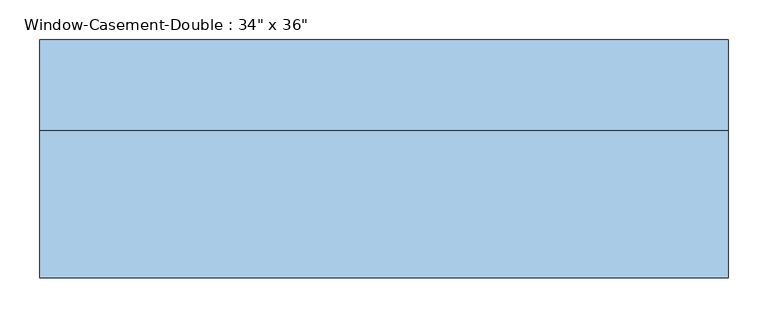
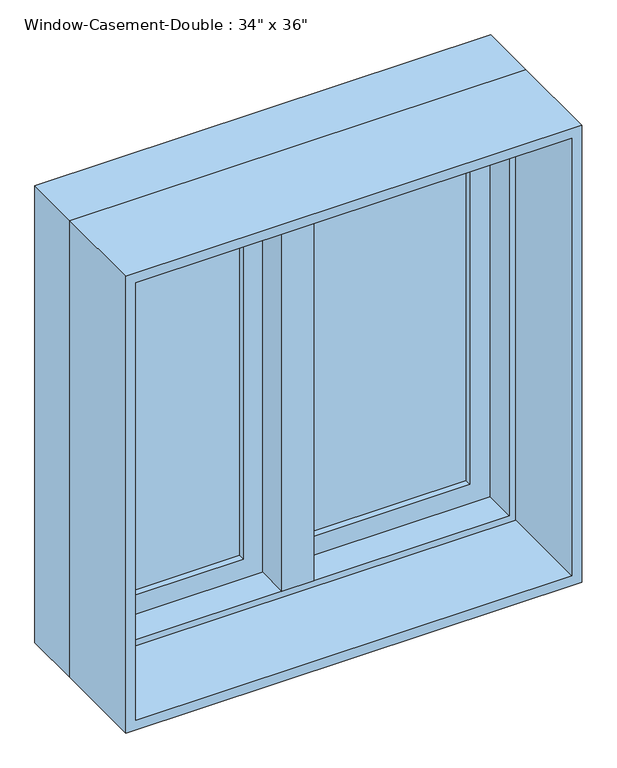
"""IFC4 building model written with IfcOpenShell, lengths in millimetres: window geometry."""

from ifc_helpers import new_model, si_unit, frame, origin, place, context, project, spatial, polyline, outline, extrude, faceted_brep, source, transform, mapped, element, save


def window_6eb120d7(model_context):
    return source(origin(), model_context, "Body", "SolidModel", [
        faceted_brep([(9.525, 158.75, 1816.1), (-9.525, 158.75, 1816.1), (-9.525, 107.95, 1816.1), (9.525, 107.95, 1816.1), (9.525, 158.75, 927.1), (9.525, 107.95, 927.1), (-9.525, 107.95, 927.1), (-9.525, 158.75, 927.1), (-9.525, 107.95, 946.15), (-9.525, 107.95, 1797.05), (-30.1625, 107.95, 946.15), (-30.1625, 107.95, 1797.05), (-30.1625, 44.45, 946.15), (-30.1625, 44.45, 1797.05), (30.1625, 44.45, 946.15), (30.1625, 44.45, 1797.05), (30.1625, 107.95, 946.15), (30.1625, 107.95, 1797.05), (9.525, 107.95, 946.15), (9.525, 107.95, 1797.05)], [[[0, 1, 2, 3]], [[4, 5, 6, 7]], [[1, 0, 4, 7]], [[2, 1, 7, 6, 8, 9]], [[9, 8, 10, 11]], [[11, 10, 12, 13]], [[13, 12, 14, 15]], [[15, 14, 16, 17]], [[17, 16, 18, 19]], [[0, 3, 19, 18, 5, 4]], [[18, 8, 6, 5]], [[9, 19, 3, 2]], [[8, 18, 16, 14, 12, 10]], [[19, 9, 11, 13, 15, 17]]]),
        extrude(outline(polyline([(-66.675, 139.7), (-66.675, 133.35), (-361.95, 133.35), (-361.95, 139.7), (-66.675, 139.7)])), frame((0.0, 0.0, 984.25), z_axis=(0.0, 0.0, 1.0), x_axis=(1.0, 0.0, 0.0)), (0.0, 0.0, 1.0), 774.7),
        extrude(outline(polyline([(-361.95, 120.65), (-361.95, 127.0), (-66.675, 127.0), (-66.675, 120.65), (-361.95, 120.65)])), frame((0.0, 0.0, 984.25), z_axis=(0.0, 0.0, 1.0), x_axis=(1.0, 0.0, 0.0)), (0.0, 0.0, 1.0), 774.7),
        extrude(outline(polyline([(361.95, 139.7), (361.95, 133.35), (66.675, 133.35), (66.675, 139.7), (361.95, 139.7)])), frame((0.0, 0.0, 984.25), z_axis=(0.0, 0.0, 1.0), x_axis=(1.0, 0.0, 0.0)), (0.0, 0.0, 1.0), 774.7),
        extrude(outline(polyline([(66.675, 120.65), (66.675, 127.0), (361.95, 127.0), (361.95, 120.65), (66.675, 120.65)])), frame((0.0, 0.0, 984.25), z_axis=(0.0, 0.0, 1.0), x_axis=(1.0, 0.0, 0.0)), (0.0, 0.0, 1.0), 774.7),
        extrude(outline(polyline([(1816.1, -419.1), (927.1, -419.1), (927.1, -9.525), (1816.1, -9.525), (1816.1, -419.1)]), holes=[polyline([(1758.95, -66.675), (984.25, -66.675), (984.25, -361.95), (1758.95, -361.95), (1758.95, -66.675)])]), frame((0.0, 107.95, 0.0), z_axis=(0.0, 1.0, 0.0), x_axis=(0.0, 0.0, 1.0)), (0.0, 0.0, 1.0), 44.45),
        extrude(outline(polyline([(927.1, 419.1), (1816.1, 419.1), (1816.1, 9.525), (927.1, 9.525), (927.1, 419.1)]), holes=[polyline([(984.25, 66.675), (1758.95, 66.675), (1758.95, 361.95), (984.25, 361.95), (984.25, 66.675)])]), frame((0.0, 107.95, 0.0), z_axis=(0.0, 1.0, 0.0), x_axis=(0.0, 0.0, 1.0)), (0.0, 0.0, 1.0), 44.45),
        extrude(outline(polyline([(1828.8, -431.8), (914.4, -431.8), (914.4, 431.8), (1828.8, 431.8), (1828.8, -431.8)]), holes=[polyline([(1809.75, 412.75), (933.45, 412.75), (933.45, -412.75), (1809.75, -412.75), (1809.75, 412.75)])]), frame((0.0, -139.7, 0.0), z_axis=(0.0, 1.0, 0.0), x_axis=(0.0, 0.0, 1.0)), (0.0, 0.0, 1.0), 184.15),
        faceted_brep([(400.05, 107.95, 1797.05), (400.05, 44.45, 1797.05), (-400.05, 44.45, 1797.05), (-400.05, 107.95, 1797.05), (419.1, 158.75, 1816.1), (419.1, 107.95, 1816.1), (-419.1, 107.95, 1816.1), (-419.1, 158.75, 1816.1), (431.8, 44.45, 1828.8), (431.8, 158.75, 1828.8), (-431.8, 158.75, 1828.8), (-431.8, 44.45, 1828.8), (-400.05, 44.45, 946.15), (-400.05, 107.95, 946.15), (-419.1, 107.95, 927.1), (-419.1, 158.75, 927.1), (-431.8, 158.75, 914.4), (-431.8, 44.45, 914.4), (400.05, 44.45, 946.15), (400.05, 107.95, 946.15), (419.1, 107.95, 927.1), (419.1, 158.75, 927.1), (431.8, 158.75, 914.4), (431.8, 44.45, 914.4)], [[[0, 1, 2, 3]], [[4, 5, 6, 7]], [[8, 9, 10, 11]], [[3, 2, 12, 13]], [[7, 6, 14, 15]], [[11, 10, 16, 17]], [[13, 12, 18, 19]], [[15, 14, 20, 21]], [[17, 16, 22, 23]], [[11, 17, 23, 8], [1, 18, 12, 2]], [[19, 18, 1, 0]], [[5, 20, 14, 6], [3, 13, 19, 0]], [[21, 20, 5, 4]], [[23, 22, 9, 8]], [[9, 22, 16, 10], [7, 15, 21, 4]]]),
    ])


if __name__ == "__main__":
    model = new_model("IFC4")
    model_context = context("Model", 3, world=origin())
    ifc_project = project(units=[si_unit("LENGTHUNIT", "METRE", prefix="MILLI")], contexts=[model_context])
    site = spatial("IfcSite", under=ifc_project)
    building = spatial("IfcBuilding", under=site)
    placement = place(None, origin())
    window_shape = window_6eb120d7(model_context)
    element("IfcWindow", 1, ObjectType="Window-Casement-Double : 34\" x 36\"", at=placement, inside=building, context=model_context, shape_type="MappedRepresentation", body=[
        mapped(window_shape, transform((0.0, 0.0, 0.0), x_axis=(1.0, 0.0, 0.0), y_axis=(0.0, 1.0, 0.0), z_axis=(0.0, 0.0, 1.0))),
    ])
    save(model, "model.ifc")

# Revit data of these elements
# Type "Window-Casement-Double : 34\" x 36\""
#   Type Mark = "14"
#   Fire Rating = "0.5h"
#   Assembly Code = "B2020100"
#   Analytic Construction = "Double glazing - domestic"
#   Frame Extension [instance default] = 0.25"
#   Window Inset [instance default] = 0"
#   Wall Thickness [instance default] = 6"
#   Interior Wall Closure [instance default] = 2.25"
#   Half Width = 17"
#   Visual Light Transmittance = 0.81
#   Thermal Resistance (R) = 1.8146 (h·ft²·°F)/BTU
#   Solar Heat Gain Coefficient = 0.76
#   Rough Width = 34.5"
#   Rough Height = 36.5"
#   Height = 36"
#   Heat Transfer Coefficient (U) = 0.5511 BTU/(h·ft²·°F)
#   Exterior Wall Closure [instance default] = 1.25"
#   Extension Jamb [instance default] = 2.25"
#   Default Sill Height = 36"
#   Width = 34"
#   Define Thermal Properties by = 0
#   Muntin Visibility = yes
#   Interior Trim Visibility [instance default] = yes
#   Exterior Trim Visibility [instance default] = yes
#   Extension Jamb Visibility [instance default] = yes
#   Interior Trim Material = Wood - Stained
#   Muntin Pattern = Muntin Pattern_2x2 : Muntin Pattern_2x2
#   Interior Trim = Trim-Window-Interior-Flat : Picture Frame
#   Interior Frame Material = Wood - Stained
#   Glass Panel Material = Glass
#   Exterior Trim Material = Clad - White
#   Exterior Trim = Trim-Window-Exterior-Flat : with Sill
#   Exterior Frame Material = Clad - White
#   Wall Closure = (empty or 0)
# Element 1 (IfcWindow, "Window-Casement-Double : 34\" x 36\"")
#   Wall Thickness = 11"
#   Extension Jamb = 7.25"
#   Materials on its faces: "Wood - Stained", "Glass", "Clad - White"
# Materials
#   "Wood - Stained": class "Wood", colour RGB 224 178 126, transparency 0, Cost = 0
#   "Glass": class "Glass", colour RGB 0 128 192, transparency 0.75, Description = "Soda Lime Glass", Cost = 0
#   "Clad - White": class "Wood", colour RGB 242 242 238, transparency 0, Cost = 0
